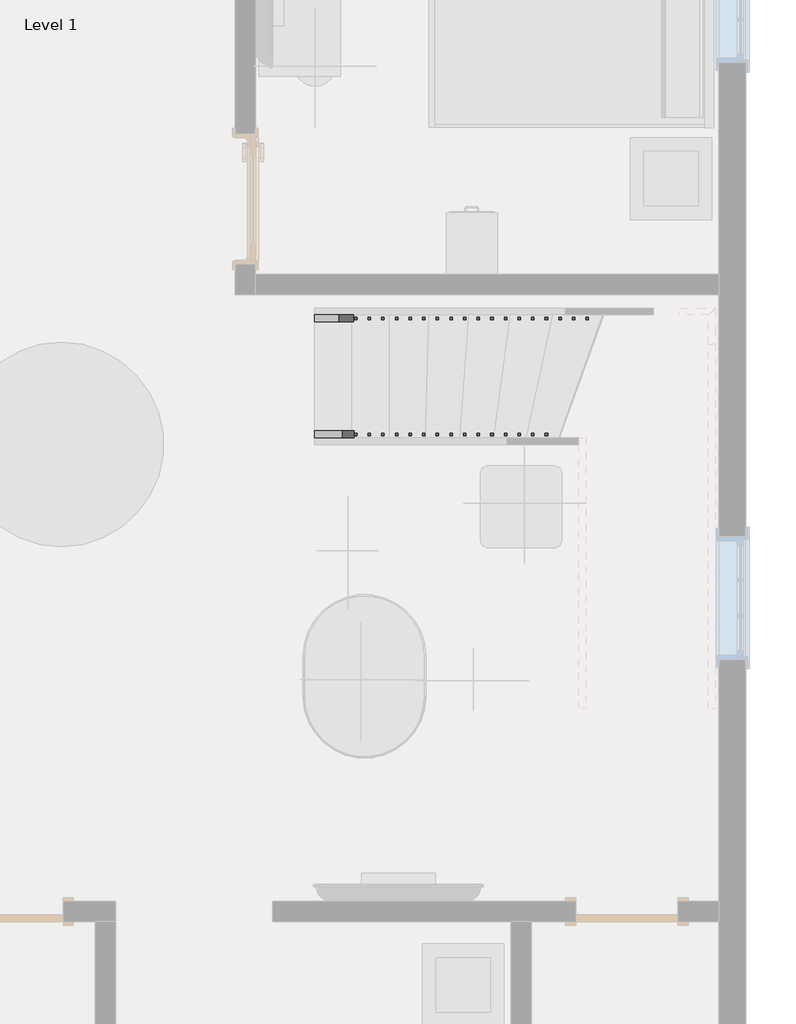
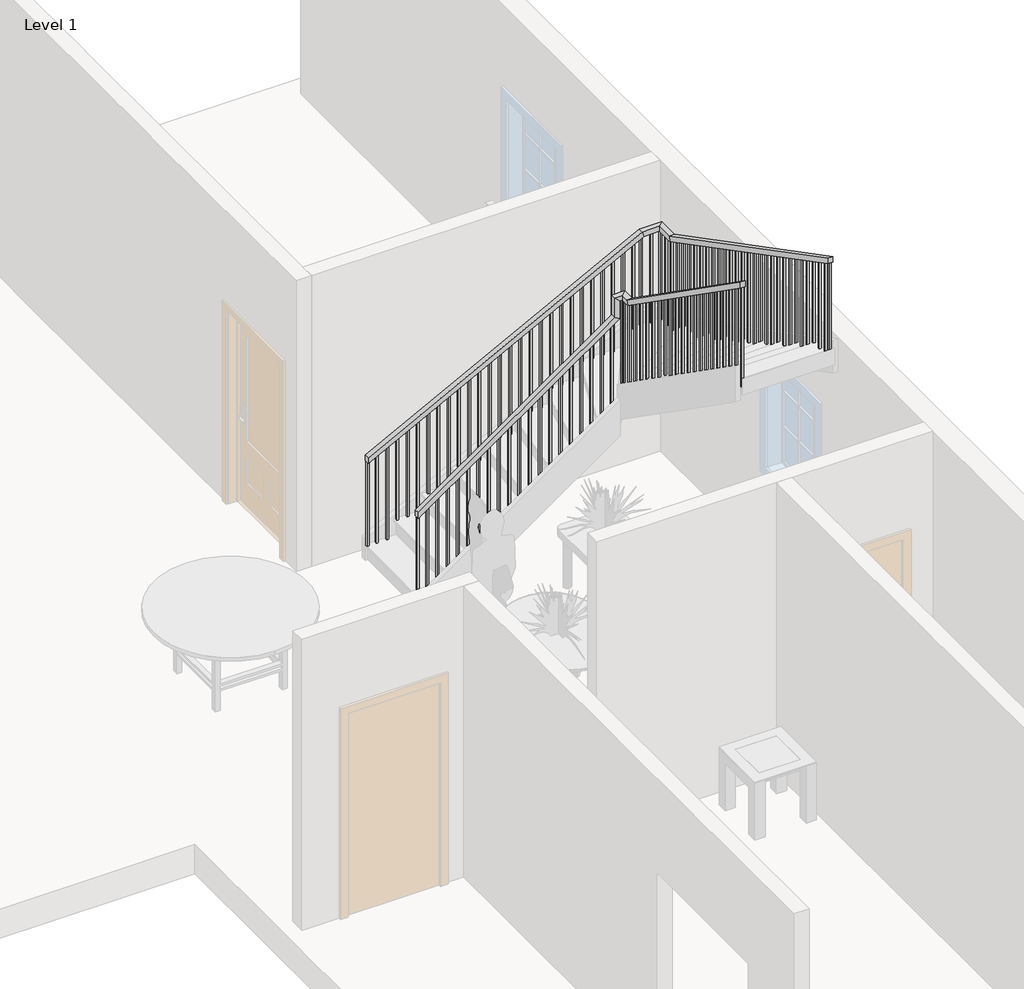
# One storey, part 3 of 4: 2 railings.
"""IFC4 building model written with IfcOpenShell, lengths in millimetres."""

from ifc_helpers import new_model, si_unit, frame, origin, place, context, project, spatial, polyline, outline, extrude, faceted_brep, element, save

model = new_model("IFC4")

# Units and contexts
model_context = context("Model", 3, world=origin())
ifc_project = project(units=[si_unit("LENGTHUNIT", "METRE", prefix="MILLI")], contexts=[model_context])

# Site, building, storey
site = spatial("IfcSite", under=ifc_project)
building = spatial("IfcBuilding", under=site)
storey = spatial("IfcBuildingStorey", under=building, Name="Level 1", Elevation=0.0)

# Railings
placement = place(None, origin())
element("IfcRailing", 1, ObjectType="Handrail - Rectangular", at=placement, inside=storey, context=model_context, shape_type="SolidModel", body=[
    faceted_brep([(-5670.2346501, 6461.8271763, 1057.2428855), (-5670.2346501, 6461.8271763, 995.2081543), (-5670.2346501, 6411.0271763, 995.2081543), (-5670.2346501, 6411.0271763, 1057.2428855), (-3724.8976606, 6461.8271763, 2420.6761173), (-3674.0976606, 6461.8271763, 2394.2457099), (-3674.0976606, 6411.0271763, 2394.2457099), (-3724.8976606, 6411.0271763, 2420.6761173), (-3724.8976606, 6461.8271763, 2625.457216), (-3674.0976606, 6461.8271763, 2574.657216), (-3674.0976606, 6411.0271763, 2574.657216), (-3724.8976606, 6411.0271763, 2625.457216), (-3597.8976606, 6461.8271763, 2625.457216), (-3597.8976606, 6461.8271763, 2574.657216), (-3648.6976606, 6411.0271763, 2574.657216), (-3648.6976606, 6411.0271763, 2625.457216), (-3597.8976606, 6334.8271763, 2625.457216), (-3597.8976606, 6318.7975404, 2574.657216), (-3648.6976606, 6318.7975404, 2574.657216), (-3648.6976606, 6334.8271763, 2625.457216), (-3597.8976606, 4389.4901868, 3988.8904479), (-3648.6976606, 4389.4901868, 3988.8904479), (-3648.6976606, 4389.4901868, 3926.8557166), (-3597.8976606, 4389.4901868, 3926.8557166)], [[[0, 1, 2, 3]], [[1, 0, 4, 5]], [[2, 1, 5, 6]], [[3, 2, 6, 7]], [[0, 3, 7, 4]], [[5, 4, 8, 9]], [[6, 5, 9, 10]], [[7, 6, 10, 11]], [[4, 7, 11, 8]], [[9, 8, 12, 13]], [[10, 9, 13, 14]], [[11, 10, 14, 15]], [[8, 11, 15, 12]], [[13, 12, 16, 17]], [[14, 13, 17, 18]], [[15, 14, 18, 19]], [[12, 15, 19, 16]], [[20, 21, 22, 23]], [[17, 16, 20, 23]], [[18, 17, 23, 22]], [[19, 18, 22, 21]], [[16, 19, 21, 20]]]),
    extrude(outline(polyline([(4394.9021763, 3923.0626019), (4413.9521763, 3909.7109805), (4413.9521763, 2878.6666667), (4394.9021763, 2878.6666667), (4394.9021763, 3923.0626019)])), frame((-3632.8226606, 0.0, 0.0), z_axis=(1.0, 0.0, 0.0), x_axis=(0.0, 1.0, 0.0)), (0.0, 0.0, 1.0), 19.05),
    extrude(outline(polyline([(4496.5021763, 3851.8539542), (4515.5521763, 3838.5023328), (4515.5521763, 2878.6666667), (4496.5021763, 2878.6666667), (4496.5021763, 3851.8539542)])), frame((-3632.8226606, 0.0, 0.0), z_axis=(1.0, 0.0, 0.0), x_axis=(0.0, 1.0, 0.0)), (0.0, 0.0, 1.0), 19.05),
    extrude(outline(polyline([(4598.1021763, 3780.7235858), (4617.1521763, 3767.3719643), (4617.1521763, 2878.6666667), (4598.1021763, 2878.6666667), (4598.1021763, 3780.7235858)])), frame((-3632.8226606, 0.0, 0.0), z_axis=(1.0, 0.0, 0.0), x_axis=(0.0, 1.0, 0.0)), (0.0, 0.0, 1.0), 19.05),
    extrude(outline(polyline([(4699.7021763, 3709.514938), (4718.7521763, 3696.1633166), (4718.7521763, 2709.3333333), (4699.7021763, 2709.3333333), (4699.7021763, 3709.514938)])), frame((-3632.8226606, 0.0, 0.0), z_axis=(1.0, 0.0, 0.0), x_axis=(0.0, 1.0, 0.0)), (0.0, 0.0, 1.0), 19.05),
    extrude(outline(polyline([(4801.3021763, 3638.3062903), (4820.3521763, 3624.9546689), (4820.3521763, 2709.3333333), (4801.3021763, 2709.3333333), (4801.3021763, 3638.3062903)])), frame((-3632.8226606, 0.0, 0.0), z_axis=(1.0, 0.0, 0.0), x_axis=(0.0, 1.0, 0.0)), (0.0, 0.0, 1.0), 19.05),
    extrude(outline(polyline([(4902.9021763, 3567.0193634), (4921.9521763, 3553.667742), (4921.9521763, 2709.3333333), (4902.9021763, 2709.3333333), (4902.9021763, 3567.0193634)])), frame((-3632.8226606, 0.0, 0.0), z_axis=(1.0, 0.0, 0.0), x_axis=(0.0, 1.0, 0.0)), (0.0, 0.0, 1.0), 19.05),
    extrude(outline(polyline([(5004.5021763, 3495.8889949), (5023.5521763, 3482.5373735), (5023.5521763, 2540.0), (5004.5021763, 2540.0), (5004.5021763, 3495.8889949)])), frame((-3632.8226606, 0.0, 0.0), z_axis=(1.0, 0.0, 0.0), x_axis=(0.0, 1.0, 0.0)), (0.0, 0.0, 1.0), 19.05),
    extrude(outline(polyline([(5106.1021763, 3424.602068), (5125.1521763, 3411.2504466), (5125.1521763, 2540.0), (5106.1021763, 2540.0), (5106.1021763, 3424.602068)])), frame((-3632.8226606, 0.0, 0.0), z_axis=(1.0, 0.0, 0.0), x_axis=(0.0, 1.0, 0.0)), (0.0, 0.0, 1.0), 19.05),
    extrude(outline(polyline([(5207.7021763, 3353.4716995), (5226.7521763, 3340.1200781), (5226.7521763, 2370.6666667), (5207.7021763, 2370.6666667), (5207.7021763, 3353.4716995)])), frame((-3632.8226606, 0.0, 0.0), z_axis=(1.0, 0.0, 0.0), x_axis=(0.0, 1.0, 0.0)), (0.0, 0.0, 1.0), 19.05),
    extrude(outline(polyline([(5309.3021763, 3282.1847726), (5328.3521763, 3268.8331511), (5328.3521763, 2370.6666667), (5309.3021763, 2370.6666667), (5309.3021763, 3282.1847726)])), frame((-3632.8226606, 0.0, 0.0), z_axis=(1.0, 0.0, 0.0), x_axis=(0.0, 1.0, 0.0)), (0.0, 0.0, 1.0), 19.05),
    extrude(outline(polyline([(5410.9021763, 3210.9761249), (5429.9521763, 3197.6245034), (5429.9521763, 2370.6666667), (5410.9021763, 2370.6666667), (5410.9021763, 3210.9761249)])), frame((-3632.8226606, 0.0, 0.0), z_axis=(1.0, 0.0, 0.0), x_axis=(0.0, 1.0, 0.0)), (0.0, 0.0, 1.0), 19.05),
    extrude(outline(polyline([(5512.5021763, 3139.8457564), (5531.5521763, 3126.494135), (5531.5521763, 2201.3333333), (5512.5021763, 2201.3333333), (5512.5021763, 3139.8457564)])), frame((-3632.8226606, 0.0, 0.0), z_axis=(1.0, 0.0, 0.0), x_axis=(0.0, 1.0, 0.0)), (0.0, 0.0, 1.0), 19.05),
    extrude(outline(polyline([(5614.1021763, 3068.5588295), (5633.1521763, 3055.207208), (5633.1521763, 2201.3333333), (5614.1021763, 2201.3333333), (5614.1021763, 3068.5588295)])), frame((-3632.8226606, 0.0, 0.0), z_axis=(1.0, 0.0, 0.0), x_axis=(0.0, 1.0, 0.0)), (0.0, 0.0, 1.0), 19.05),
    extrude(outline(polyline([(5715.7021763, 2997.3501818), (5734.7521763, 2983.9985603), (5734.7521763, 2201.3333333), (5715.7021763, 2201.3333333), (5715.7021763, 2997.3501818)])), frame((-3632.8226606, 0.0, 0.0), z_axis=(1.0, 0.0, 0.0), x_axis=(0.0, 1.0, 0.0)), (0.0, 0.0, 1.0), 19.05),
    extrude(outline(polyline([(5817.3021763, 2926.1415341), (5836.3521763, 2912.7899126), (5836.3521763, 2032.0), (5817.3021763, 2032.0), (5817.3021763, 2926.1415341)])), frame((-3632.8226606, 0.0, 0.0), z_axis=(1.0, 0.0, 0.0), x_axis=(0.0, 1.0, 0.0)), (0.0, 0.0, 1.0), 19.05),
    extrude(outline(polyline([(5918.9021763, 2854.9328864), (5937.9521763, 2841.5812649), (5937.9521763, 2032.0), (5918.9021763, 2032.0), (5918.9021763, 2854.9328864)])), frame((-3632.8226606, 0.0, 0.0), z_axis=(1.0, 0.0, 0.0), x_axis=(0.0, 1.0, 0.0)), (0.0, 0.0, 1.0), 19.05),
    extrude(outline(polyline([(6020.5021763, 2783.8025179), (6039.5521763, 2770.4508964), (6039.5521763, 1862.6666667), (6020.5021763, 1862.6666667), (6020.5021763, 2783.8025179)])), frame((-3632.8226606, 0.0, 0.0), z_axis=(1.0, 0.0, 0.0), x_axis=(0.0, 1.0, 0.0)), (0.0, 0.0, 1.0), 19.05),
    extrude(outline(polyline([(6122.1021763, 2712.515591), (6141.1521763, 2699.1639695), (6141.1521763, 1862.6666667), (6122.1021763, 1862.6666667), (6122.1021763, 2712.515591)])), frame((-3632.8226606, 0.0, 0.0), z_axis=(1.0, 0.0, 0.0), x_axis=(0.0, 1.0, 0.0)), (0.0, 0.0, 1.0), 19.05),
    extrude(outline(polyline([(6223.7021763, 2641.3852225), (6242.7521763, 2628.033601), (6242.7521763, 1693.3333333), (6223.7021763, 1693.3333333), (6223.7021763, 2641.3852225)])), frame((-3632.8226606, 0.0, 0.0), z_axis=(1.0, 0.0, 0.0), x_axis=(0.0, 1.0, 0.0)), (0.0, 0.0, 1.0), 19.05),
    extrude(outline(polyline([(-3632.8226606, 6344.3521763), (-3613.7726606, 6344.3521763), (-3613.7726606, 6325.3021763), (-3632.8226606, 6325.3021763), (-3632.8226606, 6344.3521763)])), frame((0.0, 0.0, 1693.3333333), z_axis=(0.0, 0.0, 1.0), x_axis=(1.0, 0.0, 0.0)), (0.0, 0.0, 1.0), 881.3238827),
    extrude(outline(polyline([(-3647.7596501, 6426.9021763), (-3647.7596501, 6445.9521763), (-3628.7096501, 6445.9521763), (-3628.7096501, 6426.9021763), (-3647.7596501, 6426.9021763)])), frame((0.0, 0.0, 1524.0), z_axis=(0.0, 0.0, 1.0), x_axis=(1.0, 0.0, 0.0)), (0.0, 0.0, 1.0), 1050.657216),
    extrude(outline(polyline([(2354.8482714, -3730.3096501), (2341.4966499, -3749.3596501), (1354.6666667, -3749.3596501), (1354.6666667, -3730.3096501), (2354.8482714, -3730.3096501)])), frame((0.0, 6426.9021763, 0.0), z_axis=(0.0, 1.0, 0.0), x_axis=(0.0, 0.0, 1.0)), (0.0, 0.0, 1.0), 19.05),
    extrude(outline(polyline([(2283.6396237, -3831.9096501), (2270.2880022, -3850.9596501), (1354.6666667, -3850.9596501), (1354.6666667, -3831.9096501), (2283.6396237, -3831.9096501)])), frame((0.0, 6426.9021763, 0.0), z_axis=(0.0, 1.0, 0.0), x_axis=(0.0, 0.0, 1.0)), (0.0, 0.0, 1.0), 19.05),
    extrude(outline(polyline([(2212.430976, -3933.5096501), (2199.0793545, -3952.5596501), (1185.3333333, -3952.5596501), (1185.3333333, -3933.5096501), (2212.430976, -3933.5096501)])), frame((0.0, 6426.9021763, 0.0), z_axis=(0.0, 1.0, 0.0), x_axis=(0.0, 0.0, 1.0)), (0.0, 0.0, 1.0), 19.05),
    extrude(outline(polyline([(2141.2223283, -4035.1096501), (2127.8707068, -4054.1596501), (1185.3333333, -4054.1596501), (1185.3333333, -4035.1096501), (2141.2223283, -4035.1096501)])), frame((0.0, 6426.9021763, 0.0), z_axis=(0.0, 1.0, 0.0), x_axis=(0.0, 0.0, 1.0)), (0.0, 0.0, 1.0), 19.05),
    extrude(outline(polyline([(2070.0136806, -4136.7096501), (2056.6620591, -4155.7596501), (1016.0, -4155.7596501), (1016.0, -4136.7096501), (2070.0136806, -4136.7096501)])), frame((0.0, 6426.9021763, 0.0), z_axis=(0.0, 1.0, 0.0), x_axis=(0.0, 0.0, 1.0)), (0.0, 0.0, 1.0), 19.05),
    extrude(outline(polyline([(1998.8050329, -4238.3096501), (1985.4534114, -4257.3596501), (1016.0, -4257.3596501), (1016.0, -4238.3096501), (1998.8050329, -4238.3096501)])), frame((0.0, 6426.9021763, 0.0), z_axis=(0.0, 1.0, 0.0), x_axis=(0.0, 0.0, 1.0)), (0.0, 0.0, 1.0), 19.05),
    extrude(outline(polyline([(1927.5963851, -4339.9096501), (1914.2447637, -4358.9596501), (846.6666667, -4358.9596501), (846.6666667, -4339.9096501), (1927.5963851, -4339.9096501)])), frame((0.0, 6426.9021763, 0.0), z_axis=(0.0, 1.0, 0.0), x_axis=(0.0, 0.0, 1.0)), (0.0, 0.0, 1.0), 19.05),
    extrude(outline(polyline([(1856.3877374, -4441.5096501), (1843.036116, -4460.5596501), (846.6666667, -4460.5596501), (846.6666667, -4441.5096501), (1856.3877374, -4441.5096501)])), frame((0.0, 6426.9021763, 0.0), z_axis=(0.0, 1.0, 0.0), x_axis=(0.0, 0.0, 1.0)), (0.0, 0.0, 1.0), 19.05),
    extrude(outline(polyline([(1785.1790897, -4543.1096501), (1771.8274683, -4562.1596501), (846.6666667, -4562.1596501), (846.6666667, -4543.1096501), (1785.1790897, -4543.1096501)])), frame((0.0, 6426.9021763, 0.0), z_axis=(0.0, 1.0, 0.0), x_axis=(0.0, 0.0, 1.0)), (0.0, 0.0, 1.0), 19.05),
    extrude(outline(polyline([(1713.970442, -4644.7096501), (1700.6188206, -4663.7596501), (677.3333333, -4663.7596501), (677.3333333, -4644.7096501), (1713.970442, -4644.7096501)])), frame((0.0, 6426.9021763, 0.0), z_axis=(0.0, 1.0, 0.0), x_axis=(0.0, 0.0, 1.0)), (0.0, 0.0, 1.0), 19.05),
    extrude(outline(polyline([(1642.7617943, -4746.3096501), (1629.4101729, -4765.3596501), (677.3333333, -4765.3596501), (677.3333333, -4746.3096501), (1642.7617943, -4746.3096501)])), frame((0.0, 6426.9021763, 0.0), z_axis=(0.0, 1.0, 0.0), x_axis=(0.0, 0.0, 1.0)), (0.0, 0.0, 1.0), 19.05),
    extrude(outline(polyline([(1571.5531466, -4847.9096501), (1558.2015252, -4866.9596501), (508.0, -4866.9596501), (508.0, -4847.9096501), (1571.5531466, -4847.9096501)])), frame((0.0, 6426.9021763, 0.0), z_axis=(0.0, 1.0, 0.0), x_axis=(0.0, 0.0, 1.0)), (0.0, 0.0, 1.0), 19.05),
    extrude(outline(polyline([(1500.3444989, -4949.5096501), (1486.9928775, -4968.5596501), (508.0, -4968.5596501), (508.0, -4949.5096501), (1500.3444989, -4949.5096501)])), frame((0.0, 6426.9021763, 0.0), z_axis=(0.0, 1.0, 0.0), x_axis=(0.0, 0.0, 1.0)), (0.0, 0.0, 1.0), 19.05),
    extrude(outline(polyline([(1429.1358512, -5051.1096501), (1415.7842298, -5070.1596501), (508.0, -5070.1596501), (508.0, -5051.1096501), (1429.1358512, -5051.1096501)])), frame((0.0, 6426.9021763, 0.0), z_axis=(0.0, 1.0, 0.0), x_axis=(0.0, 0.0, 1.0)), (0.0, 0.0, 1.0), 19.05),
    extrude(outline(polyline([(1357.9272035, -5152.7096501), (1344.5755821, -5171.7596501), (338.6666667, -5171.7596501), (338.6666667, -5152.7096501), (1357.9272035, -5152.7096501)])), frame((0.0, 6426.9021763, 0.0), z_axis=(0.0, 1.0, 0.0), x_axis=(0.0, 0.0, 1.0)), (0.0, 0.0, 1.0), 19.05),
    extrude(outline(polyline([(1286.7185558, -5254.3096501), (1273.3669344, -5273.3596501), (338.6666667, -5273.3596501), (338.6666667, -5254.3096501), (1286.7185558, -5254.3096501)])), frame((0.0, 6426.9021763, 0.0), z_axis=(0.0, 1.0, 0.0), x_axis=(0.0, 0.0, 1.0)), (0.0, 0.0, 1.0), 19.05),
    extrude(outline(polyline([(1215.5099081, -5355.9096501), (1202.1582867, -5374.9596501), (338.6666667, -5374.9596501), (338.6666667, -5355.9096501), (1215.5099081, -5355.9096501)])), frame((0.0, 6426.9021763, 0.0), z_axis=(0.0, 1.0, 0.0), x_axis=(0.0, 0.0, 1.0)), (0.0, 0.0, 1.0), 19.05),
    extrude(outline(polyline([(1144.2229812, -5457.5096501), (1130.8713597, -5476.5596501), (169.3333333, -5476.5596501), (169.3333333, -5457.5096501), (1144.2229812, -5457.5096501)])), frame((0.0, 6426.9021763, 0.0), z_axis=(0.0, 1.0, 0.0), x_axis=(0.0, 0.0, 1.0)), (0.0, 0.0, 1.0), 19.05),
    extrude(outline(polyline([(1073.0926127, -5559.1096501), (1059.7409912, -5578.1596501), (169.3333333, -5578.1596501), (169.3333333, -5559.1096501), (1073.0926127, -5559.1096501)])), frame((0.0, 6426.9021763, 0.0), z_axis=(0.0, 1.0, 0.0), x_axis=(0.0, 0.0, 1.0)), (0.0, 0.0, 1.0), 19.05),
    extrude(outline(polyline([(-3632.8226606, 6445.9521763), (-3613.7726606, 6445.9521763), (-3613.7726606, 6426.9021763), (-3632.8226606, 6426.9021763), (-3632.8226606, 6445.9521763)])), frame((0.0, 0.0, 1524.0), z_axis=(0.0, 0.0, 1.0), x_axis=(1.0, 0.0, 0.0)), (0.0, 0.0, 1.0), 1050.657216),
    extrude(outline(polyline([(4389.4901868, 3926.8557166), (4408.5401868, 3913.5040952), (4408.5401868, 2878.6666667), (4389.4901868, 2878.6666667), (4389.4901868, 3926.8557166)])), frame((-3632.8226606, 0.0, 0.0), z_axis=(1.0, 0.0, 0.0), x_axis=(0.0, 1.0, 0.0)), (0.0, 0.0, 1.0), 19.05),
    extrude(outline(polyline([(1008.5597757, -5651.1846501), (995.2081543, -5670.2346501), (169.3333333, -5670.2346501), (169.3333333, -5651.1846501), (1008.5597757, -5651.1846501)])), frame((0.0, 6426.9021763, 0.0), z_axis=(0.0, 1.0, 0.0), x_axis=(0.0, 0.0, 1.0)), (0.0, 0.0, 1.0), 19.05),
])
element("IfcRailing", 2, ObjectType="Handrail - Rectangular", at=placement, inside=storey, context=model_context, shape_type="SolidModel", body=[
    faceted_brep([(-5670.2346501, 7325.4271763, 1107.5448574), (-5670.2346501, 7325.4271763, 1050.2675251), (-5670.2346501, 7274.6271763, 1050.2675251), (-5670.2346501, 7274.6271763, 1107.5448574), (-2952.4510037, 7325.4271763, 2523.0666667), (-2940.0146092, 7325.4271763, 2472.2666667), (-2940.0146092, 7274.6271763, 2472.2666667), (-2952.4510037, 7274.6271763, 2523.0666667), (-2734.2976606, 7325.4271763, 2523.0666667), (-2734.2976606, 7325.4271763, 2472.2666667), (-2785.0976606, 7274.6271763, 2472.2666667), (-2785.0976606, 7274.6271763, 2523.0666667), (-2734.2976606, 7107.2738332, 2523.0666667), (-2734.2976606, 7094.8374386, 2472.2666667), (-2785.0976606, 7094.8374386, 2472.2666667), (-2785.0976606, 7107.2738332, 2523.0666667), (-2734.2976606, 4389.4901868, 3938.588476), (-2785.0976606, 4389.4901868, 3938.588476), (-2785.0976606, 4389.4901868, 3881.3111437), (-2734.2976606, 4389.4901868, 3881.3111437)], [[[0, 1, 2, 3]], [[1, 0, 4, 5]], [[2, 1, 5, 6]], [[3, 2, 6, 7]], [[0, 3, 7, 4]], [[5, 4, 8, 9]], [[6, 5, 9, 10]], [[7, 6, 10, 11]], [[4, 7, 11, 8]], [[9, 8, 12, 13]], [[10, 9, 13, 14]], [[11, 10, 14, 15]], [[8, 11, 15, 12]], [[16, 17, 18, 19]], [[13, 12, 16, 19]], [[14, 13, 19, 18]], [[15, 14, 18, 17]], [[12, 15, 17, 16]]]),
    extrude(outline(polyline([(4475.1988332, 3836.6652459), (4475.1988332, 2878.6666667), (4456.1488332, 2878.6666667), (4456.1488332, 3846.5871875), (4475.1988332, 3836.6652459)])), frame((-2769.2226606, 0.0, 0.0), z_axis=(1.0, 0.0, 0.0), x_axis=(0.0, 1.0, 0.0)), (0.0, 0.0, 1.0), 19.05),
    extrude(outline(polyline([(4576.7988332, 3783.7539027), (4576.7988332, 2878.6666667), (4557.7488332, 2878.6666667), (4557.7488332, 3793.6758443), (4576.7988332, 3783.7539027)])), frame((-2769.2226606, 0.0, 0.0), z_axis=(1.0, 0.0, 0.0), x_axis=(0.0, 1.0, 0.0)), (0.0, 0.0, 1.0), 19.05),
    extrude(outline(polyline([(4678.3988332, 3730.8368812), (4678.3988332, 2878.6751842), (4659.3488332, 2878.6751842), (4659.3488332, 3740.7588227), (4678.3988332, 3730.8368812)])), frame((-2769.2226606, 0.0, 0.0), z_axis=(1.0, 0.0, 0.0), x_axis=(0.0, 1.0, 0.0)), (0.0, 0.0, 1.0), 19.05),
    extrude(outline(polyline([(4779.9988332, 3677.9141812), (4779.9988332, 2709.3333333), (4760.9488332, 2709.3333333), (4760.9488332, 3687.8361228), (4779.9988332, 3677.9141812)])), frame((-2769.2226606, 0.0, 0.0), z_axis=(1.0, 0.0, 0.0), x_axis=(0.0, 1.0, 0.0)), (0.0, 0.0, 1.0), 19.05),
    extrude(outline(polyline([(4881.5988332, 3624.9971597), (4881.5988332, 2709.3333333), (4862.5488332, 2709.3333333), (4862.5488332, 3634.9191012), (4881.5988332, 3624.9971597)])), frame((-2769.2226606, 0.0, 0.0), z_axis=(1.0, 0.0, 0.0), x_axis=(0.0, 1.0, 0.0)), (0.0, 0.0, 1.0), 19.05),
    extrude(outline(polyline([(4983.1988332, 3572.0801381), (4983.1988332, 2540.0), (4964.1488332, 2540.0), (4964.1488332, 3582.0020796), (4983.1988332, 3572.0801381)])), frame((-2769.2226606, 0.0, 0.0), z_axis=(1.0, 0.0, 0.0), x_axis=(0.0, 1.0, 0.0)), (0.0, 0.0, 1.0), 19.05),
    extrude(outline(polyline([(5084.7988332, 3519.1631165), (5084.7988332, 2540.0), (5065.7488332, 2540.0), (5065.7488332, 3529.0850581), (5084.7988332, 3519.1631165)])), frame((-2769.2226606, 0.0, 0.0), z_axis=(1.0, 0.0, 0.0), x_axis=(0.0, 1.0, 0.0)), (0.0, 0.0, 1.0), 19.05),
    extrude(outline(polyline([(5186.3988332, 3466.246095), (5186.3988332, 2540.0), (5167.3488332, 2540.0), (5167.3488332, 3476.1680365), (5186.3988332, 3466.246095)])), frame((-2769.2226606, 0.0, 0.0), z_axis=(1.0, 0.0, 0.0), x_axis=(0.0, 1.0, 0.0)), (0.0, 0.0, 1.0), 19.05),
    extrude(outline(polyline([(5287.9988332, 3413.3347518), (5287.9988332, 2370.6666667), (5268.9488332, 2370.6666667), (5268.9488332, 3423.2566933), (5287.9988332, 3413.3347518)])), frame((-2769.2226606, 0.0, 0.0), z_axis=(1.0, 0.0, 0.0), x_axis=(0.0, 1.0, 0.0)), (0.0, 0.0, 1.0), 19.05),
    extrude(outline(polyline([(5389.5988332, 3360.4120518), (5389.5988332, 2370.6666667), (5370.5488332, 2370.6666667), (5370.5488332, 3370.3339934), (5389.5988332, 3360.4120518)])), frame((-2769.2226606, 0.0, 0.0), z_axis=(1.0, 0.0, 0.0), x_axis=(0.0, 1.0, 0.0)), (0.0, 0.0, 1.0), 19.05),
    extrude(outline(polyline([(5491.1988332, 3307.4950303), (5491.1988332, 2370.6666667), (5472.1488332, 2370.6666667), (5472.1488332, 3317.4169718), (5491.1988332, 3307.4950303)])), frame((-2769.2226606, 0.0, 0.0), z_axis=(1.0, 0.0, 0.0), x_axis=(0.0, 1.0, 0.0)), (0.0, 0.0, 1.0), 19.05),
    extrude(outline(polyline([(5592.7988332, 3254.5836871), (5592.7988332, 2201.3333333), (5573.7488332, 2201.3333333), (5573.7488332, 3264.5056286), (5592.7988332, 3254.5836871)])), frame((-2769.2226606, 0.0, 0.0), z_axis=(1.0, 0.0, 0.0), x_axis=(0.0, 1.0, 0.0)), (0.0, 0.0, 1.0), 19.05),
    extrude(outline(polyline([(5694.3988332, 3201.6666655), (5694.3988332, 2201.3333333), (5675.3488332, 2201.3333333), (5675.3488332, 3211.5886071), (5694.3988332, 3201.6666655)])), frame((-2769.2226606, 0.0, 0.0), z_axis=(1.0, 0.0, 0.0), x_axis=(0.0, 1.0, 0.0)), (0.0, 0.0, 1.0), 19.05),
    extrude(outline(polyline([(5795.9988332, 3148.749644), (5795.9988332, 2201.3333333), (5776.9488332, 2201.3333333), (5776.9488332, 3158.6715855), (5795.9988332, 3148.749644)])), frame((-2769.2226606, 0.0, 0.0), z_axis=(1.0, 0.0, 0.0), x_axis=(0.0, 1.0, 0.0)), (0.0, 0.0, 1.0), 19.05),
    extrude(outline(polyline([(5897.5988332, 3095.8326224), (5897.5988332, 2032.0), (5878.5488332, 2032.0), (5878.5488332, 3105.7545639), (5897.5988332, 3095.8326224)])), frame((-2769.2226606, 0.0, 0.0), z_axis=(1.0, 0.0, 0.0), x_axis=(0.0, 1.0, 0.0)), (0.0, 0.0, 1.0), 19.05),
    extrude(outline(polyline([(5999.1988332, 3042.9156008), (5999.1988332, 2032.0), (5980.1488332, 2032.0), (5980.1488332, 3052.8375424), (5999.1988332, 3042.9156008)])), frame((-2769.2226606, 0.0, 0.0), z_axis=(1.0, 0.0, 0.0), x_axis=(0.0, 1.0, 0.0)), (0.0, 0.0, 1.0), 19.05),
    extrude(outline(polyline([(6100.7988332, 2989.9985793), (6100.7988332, 2032.0), (6081.7488332, 2032.0), (6081.7488332, 2999.9205208), (6100.7988332, 2989.9985793)])), frame((-2769.2226606, 0.0, 0.0), z_axis=(1.0, 0.0, 0.0), x_axis=(0.0, 1.0, 0.0)), (0.0, 0.0, 1.0), 19.05),
    extrude(outline(polyline([(6202.3988332, 2937.0815577), (6202.3988332, 1862.6666667), (6183.3488332, 1862.6666667), (6183.3488332, 2947.0034992), (6202.3988332, 2937.0815577)])), frame((-2769.2226606, 0.0, 0.0), z_axis=(1.0, 0.0, 0.0), x_axis=(0.0, 1.0, 0.0)), (0.0, 0.0, 1.0), 19.05),
    extrude(outline(polyline([(6303.9988332, 2884.1645361), (6303.9988332, 1862.6666667), (6284.9488332, 1862.6666667), (6284.9488332, 2894.0864777), (6303.9988332, 2884.1645361)])), frame((-2769.2226606, 0.0, 0.0), z_axis=(1.0, 0.0, 0.0), x_axis=(0.0, 1.0, 0.0)), (0.0, 0.0, 1.0), 19.05),
    extrude(outline(polyline([(6405.5988332, 2831.2475146), (6405.5988332, 1862.6666667), (6386.5488332, 1862.6666667), (6386.5488332, 2841.1694561), (6405.5988332, 2831.2475146)])), frame((-2769.2226606, 0.0, 0.0), z_axis=(1.0, 0.0, 0.0), x_axis=(0.0, 1.0, 0.0)), (0.0, 0.0, 1.0), 19.05),
    extrude(outline(polyline([(6507.1988332, 2778.330493), (6507.1988332, 1862.6666667), (6488.1488332, 1862.6666667), (6488.1488332, 2788.2524345), (6507.1988332, 2778.330493)])), frame((-2769.2226606, 0.0, 0.0), z_axis=(1.0, 0.0, 0.0), x_axis=(0.0, 1.0, 0.0)), (0.0, 0.0, 1.0), 19.05),
    extrude(outline(polyline([(6608.7988332, 2725.4134714), (6608.7988332, 1693.3333333), (6589.7488332, 1693.3333333), (6589.7488332, 2735.335413), (6608.7988332, 2725.4134714)])), frame((-2769.2226606, 0.0, 0.0), z_axis=(1.0, 0.0, 0.0), x_axis=(0.0, 1.0, 0.0)), (0.0, 0.0, 1.0), 19.05),
    extrude(outline(polyline([(6710.3988332, 2672.4964499), (6710.3988332, 1693.3333333), (6691.3488332, 1693.3333333), (6691.3488332, 2682.4183914), (6710.3988332, 2672.4964499)])), frame((-2769.2226606, 0.0, 0.0), z_axis=(1.0, 0.0, 0.0), x_axis=(0.0, 1.0, 0.0)), (0.0, 0.0, 1.0), 19.05),
    extrude(outline(polyline([(6811.9988332, 2619.5794283), (6811.9988332, 1693.3333333), (6792.9488332, 1693.3333333), (6792.9488332, 2629.5013699), (6811.9988332, 2619.5794283)])), frame((-2769.2226606, 0.0, 0.0), z_axis=(1.0, 0.0, 0.0), x_axis=(0.0, 1.0, 0.0)), (0.0, 0.0, 1.0), 19.05),
    extrude(outline(polyline([(6913.5988332, 2566.6624067), (6913.5988332, 1693.3333333), (6894.5488332, 1693.3333333), (6894.5488332, 2576.5843483), (6913.5988332, 2566.6624067)])), frame((-2769.2226606, 0.0, 0.0), z_axis=(1.0, 0.0, 0.0), x_axis=(0.0, 1.0, 0.0)), (0.0, 0.0, 1.0), 19.05),
    extrude(outline(polyline([(7015.1988332, 2513.7453852), (7015.1988332, 1524.0), (6996.1488332, 1524.0), (6996.1488332, 2523.6673267), (7015.1988332, 2513.7453852)])), frame((-2769.2226606, 0.0, 0.0), z_axis=(1.0, 0.0, 0.0), x_axis=(0.0, 1.0, 0.0)), (0.0, 0.0, 1.0), 19.05),
    extrude(outline(polyline([(-2750.1726606, 7207.9521763), (-2750.1726606, 7188.9021763), (-2769.2226606, 7188.9021763), (-2769.2226606, 7207.9521763), (-2750.1726606, 7207.9521763)])), frame((0.0, 0.0, 1524.0), z_axis=(0.0, 0.0, 1.0), x_axis=(1.0, 0.0, 0.0)), (0.0, 0.0, 1.0), 948.2666667),
    extrude(outline(polyline([(-2860.3760037, 7309.5521763), (-2841.3260037, 7309.5521763), (-2841.3260037, 7290.5021763), (-2860.3760037, 7290.5021763), (-2860.3760037, 7309.5521763)])), frame((0.0, 0.0, 1524.0), z_axis=(0.0, 0.0, 1.0), x_axis=(1.0, 0.0, 0.0)), (0.0, 0.0, 1.0), 948.2666667),
    extrude(outline(polyline([(2421.1434366, -3038.1596501), (1524.0, -3038.1596501), (1524.0, -3019.1096501), (2431.0653782, -3019.1096501), (2421.1434366, -3038.1596501)])), frame((0.0, 7290.5021763, 0.0), z_axis=(0.0, 1.0, 0.0), x_axis=(0.0, 0.0, 1.0)), (0.0, 0.0, 1.0), 19.05),
    extrude(outline(polyline([(2368.2264151, -3139.7596501), (1524.0, -3139.7596501), (1524.0, -3120.7096501), (2378.1483566, -3120.7096501), (2368.2264151, -3139.7596501)])), frame((0.0, 7290.5021763, 0.0), z_axis=(0.0, 1.0, 0.0), x_axis=(0.0, 0.0, 1.0)), (0.0, 0.0, 1.0), 19.05),
    extrude(outline(polyline([(2315.3093935, -3241.3596501), (1354.6666667, -3241.3596501), (1354.6666667, -3222.3096501), (2325.231335, -3222.3096501), (2315.3093935, -3241.3596501)])), frame((0.0, 7290.5021763, 0.0), z_axis=(0.0, 1.0, 0.0), x_axis=(0.0, 0.0, 1.0)), (0.0, 0.0, 1.0), 19.05),
    extrude(outline(polyline([(2262.3923719, -3342.9596501), (1354.6666667, -3342.9596501), (1354.6666667, -3323.9096501), (2272.3143135, -3323.9096501), (2262.3923719, -3342.9596501)])), frame((0.0, 7290.5021763, 0.0), z_axis=(0.0, 1.0, 0.0), x_axis=(0.0, 0.0, 1.0)), (0.0, 0.0, 1.0), 19.05),
    extrude(outline(polyline([(2209.4753504, -3444.5596501), (1354.6666667, -3444.5596501), (1354.6666667, -3425.5096501), (2219.3972919, -3425.5096501), (2209.4753504, -3444.5596501)])), frame((0.0, 7290.5021763, 0.0), z_axis=(0.0, 1.0, 0.0), x_axis=(0.0, 0.0, 1.0)), (0.0, 0.0, 1.0), 19.05),
    extrude(outline(polyline([(2156.5640072, -3546.1596501), (1354.6666667, -3546.1596501), (1354.6666667, -3527.1096501), (2166.4859487, -3527.1096501), (2156.5640072, -3546.1596501)])), frame((0.0, 7290.5021763, 0.0), z_axis=(0.0, 1.0, 0.0), x_axis=(0.0, 0.0, 1.0)), (0.0, 0.0, 1.0), 19.05),
    extrude(outline(polyline([(2103.6413072, -3647.7596501), (1185.3333333, -3647.7596501), (1185.3333333, -3628.7096501), (2113.5632488, -3628.7096501), (2103.6413072, -3647.7596501)])), frame((0.0, 7290.5021763, 0.0), z_axis=(0.0, 1.0, 0.0), x_axis=(0.0, 0.0, 1.0)), (0.0, 0.0, 1.0), 19.05),
    extrude(outline(polyline([(2050.7242857, -3749.3596501), (1185.3333333, -3749.3596501), (1185.3333333, -3730.3096501), (2060.6462272, -3730.3096501), (2050.7242857, -3749.3596501)])), frame((0.0, 7290.5021763, 0.0), z_axis=(0.0, 1.0, 0.0), x_axis=(0.0, 0.0, 1.0)), (0.0, 0.0, 1.0), 19.05),
    extrude(outline(polyline([(1997.8129425, -3850.9596501), (1185.3333333, -3850.9596501), (1185.3333333, -3831.9096501), (2007.734884, -3831.9096501), (1997.8129425, -3850.9596501)])), frame((0.0, 7290.5021763, 0.0), z_axis=(0.0, 1.0, 0.0), x_axis=(0.0, 0.0, 1.0)), (0.0, 0.0, 1.0), 19.05),
    extrude(outline(polyline([(1944.8902425, -3952.5596501), (1016.0, -3952.5596501), (1016.0, -3933.5096501), (1954.8121841, -3933.5096501), (1944.8902425, -3952.5596501)])), frame((0.0, 7290.5021763, 0.0), z_axis=(0.0, 1.0, 0.0), x_axis=(0.0, 0.0, 1.0)), (0.0, 0.0, 1.0), 19.05),
    extrude(outline(polyline([(1891.9788993, -4054.1596501), (1016.0, -4054.1596501), (1016.0, -4035.1096501), (1901.9008409, -4035.1096501), (1891.9788993, -4054.1596501)])), frame((0.0, 7290.5021763, 0.0), z_axis=(0.0, 1.0, 0.0), x_axis=(0.0, 0.0, 1.0)), (0.0, 0.0, 1.0), 19.05),
    extrude(outline(polyline([(1839.0618778, -4155.7596501), (1016.0, -4155.7596501), (1016.0, -4136.7096501), (1848.9838193, -4136.7096501), (1839.0618778, -4155.7596501)])), frame((0.0, 7290.5021763, 0.0), z_axis=(0.0, 1.0, 0.0), x_axis=(0.0, 0.0, 1.0)), (0.0, 0.0, 1.0), 19.05),
    extrude(outline(polyline([(1786.1448562, -4257.3596501), (846.6666667, -4257.3596501), (846.6666667, -4238.3096501), (1796.0667978, -4238.3096501), (1786.1448562, -4257.3596501)])), frame((0.0, 7290.5021763, 0.0), z_axis=(0.0, 1.0, 0.0), x_axis=(0.0, 0.0, 1.0)), (0.0, 0.0, 1.0), 19.05),
    extrude(outline(polyline([(1733.2278347, -4358.9596501), (846.6666667, -4358.9596501), (846.6666667, -4339.9096501), (1743.1497762, -4339.9096501), (1733.2278347, -4358.9596501)])), frame((0.0, 7290.5021763, 0.0), z_axis=(0.0, 1.0, 0.0), x_axis=(0.0, 0.0, 1.0)), (0.0, 0.0, 1.0), 19.05),
    extrude(outline(polyline([(1680.3108131, -4460.5596501), (846.6666667, -4460.5596501), (846.6666667, -4441.5096501), (1690.2327546, -4441.5096501), (1680.3108131, -4460.5596501)])), frame((0.0, 7290.5021763, 0.0), z_axis=(0.0, 1.0, 0.0), x_axis=(0.0, 0.0, 1.0)), (0.0, 0.0, 1.0), 19.05),
    extrude(outline(polyline([(1627.3937915, -4562.1596501), (677.3333333, -4562.1596501), (677.3333333, -4543.1096501), (1637.3157331, -4543.1096501), (1627.3937915, -4562.1596501)])), frame((0.0, 7290.5021763, 0.0), z_axis=(0.0, 1.0, 0.0), x_axis=(0.0, 0.0, 1.0)), (0.0, 0.0, 1.0), 19.05),
    extrude(outline(polyline([(1574.47677, -4663.7596501), (677.3333333, -4663.7596501), (677.3333333, -4644.7096501), (1584.3987115, -4644.7096501), (1574.47677, -4663.7596501)])), frame((0.0, 7290.5021763, 0.0), z_axis=(0.0, 1.0, 0.0), x_axis=(0.0, 0.0, 1.0)), (0.0, 0.0, 1.0), 19.05),
    extrude(outline(polyline([(1521.5597484, -4765.3596501), (677.3333333, -4765.3596501), (677.3333333, -4746.3096501), (1531.4816899, -4746.3096501), (1521.5597484, -4765.3596501)])), frame((0.0, 7290.5021763, 0.0), z_axis=(0.0, 1.0, 0.0), x_axis=(0.0, 0.0, 1.0)), (0.0, 0.0, 1.0), 19.05),
    extrude(outline(polyline([(1468.6427268, -4866.9596501), (508.0, -4866.9596501), (508.0, -4847.9096501), (1478.5646684, -4847.9096501), (1468.6427268, -4866.9596501)])), frame((0.0, 7290.5021763, 0.0), z_axis=(0.0, 1.0, 0.0), x_axis=(0.0, 0.0, 1.0)), (0.0, 0.0, 1.0), 19.05),
    extrude(outline(polyline([(1415.7257053, -4968.5596501), (508.0, -4968.5596501), (508.0, -4949.5096501), (1425.6476468, -4949.5096501), (1415.7257053, -4968.5596501)])), frame((0.0, 7290.5021763, 0.0), z_axis=(0.0, 1.0, 0.0), x_axis=(0.0, 0.0, 1.0)), (0.0, 0.0, 1.0), 19.05),
    extrude(outline(polyline([(1362.8086837, -5070.1596501), (508.0, -5070.1596501), (508.0, -5051.1096501), (1372.7306252, -5051.1096501), (1362.8086837, -5070.1596501)])), frame((0.0, 7290.5021763, 0.0), z_axis=(0.0, 1.0, 0.0), x_axis=(0.0, 0.0, 1.0)), (0.0, 0.0, 1.0), 19.05),
    extrude(outline(polyline([(1309.8916621, -5171.7596501), (338.6666667, -5171.7596501), (338.6666667, -5152.7096501), (1319.8136037, -5152.7096501), (1309.8916621, -5171.7596501)])), frame((0.0, 7290.5021763, 0.0), z_axis=(0.0, 1.0, 0.0), x_axis=(0.0, 0.0, 1.0)), (0.0, 0.0, 1.0), 19.05),
    extrude(outline(polyline([(1256.9746406, -5273.3596501), (338.6666667, -5273.3596501), (338.6666667, -5254.3096501), (1266.8965821, -5254.3096501), (1256.9746406, -5273.3596501)])), frame((0.0, 7290.5021763, 0.0), z_axis=(0.0, 1.0, 0.0), x_axis=(0.0, 0.0, 1.0)), (0.0, 0.0, 1.0), 19.05),
    extrude(outline(polyline([(1204.057619, -5374.9596501), (338.6666667, -5374.9596501), (338.6666667, -5355.9096501), (1213.9795606, -5355.9096501), (1204.057619, -5374.9596501)])), frame((0.0, 7290.5021763, 0.0), z_axis=(0.0, 1.0, 0.0), x_axis=(0.0, 0.0, 1.0)), (0.0, 0.0, 1.0), 19.05),
    extrude(outline(polyline([(1151.1405974, -5476.5596501), (169.3333333, -5476.5596501), (169.3333333, -5457.5096501), (1161.062539, -5457.5096501), (1151.1405974, -5476.5596501)])), frame((0.0, 7290.5021763, 0.0), z_axis=(0.0, 1.0, 0.0), x_axis=(0.0, 0.0, 1.0)), (0.0, 0.0, 1.0), 19.05),
    extrude(outline(polyline([(1098.2235759, -5578.1596501), (169.3333333, -5578.1596501), (169.3333333, -5559.1096501), (1108.1455174, -5559.1096501), (1098.2235759, -5578.1596501)])), frame((0.0, 7290.5021763, 0.0), z_axis=(0.0, 1.0, 0.0), x_axis=(0.0, 0.0, 1.0)), (0.0, 0.0, 1.0), 19.05),
    extrude(outline(polyline([(-2750.1726606, 7116.7988332), (-2750.1726606, 7097.7488332), (-2769.2226606, 7097.7488332), (-2769.2226606, 7116.7988332), (-2750.1726606, 7116.7988332)])), frame((0.0, 0.0, 1524.0), z_axis=(0.0, 0.0, 1.0), x_axis=(1.0, 0.0, 0.0)), (0.0, 0.0, 1.0), 948.2666667),
    extrude(outline(polyline([(-2769.2226606, 7309.5521763), (-2750.1726606, 7309.5521763), (-2750.1726606, 7290.5021763), (-2769.2226606, 7290.5021763), (-2769.2226606, 7309.5521763)])), frame((0.0, 0.0, 1524.0), z_axis=(0.0, 0.0, 1.0), x_axis=(1.0, 0.0, 0.0)), (0.0, 0.0, 1.0), 948.2666667),
    extrude(outline(polyline([(2460.8283636, -2961.9760037), (1524.0, -2961.9760037), (1524.0, -2942.9260037), (2470.7503052, -2942.9260037), (2460.8283636, -2961.9760037)])), frame((0.0, 7290.5021763, 0.0), z_axis=(0.0, 1.0, 0.0), x_axis=(0.0, 0.0, 1.0)), (0.0, 0.0, 1.0), 19.05),
    extrude(outline(polyline([(4408.5401868, 3871.3892021), (4408.5401868, 2878.6666667), (4389.4901868, 2878.6666667), (4389.4901868, 3881.3111437), (4408.5401868, 3871.3892021)])), frame((-2769.2226606, 0.0, 0.0), z_axis=(1.0, 0.0, 0.0), x_axis=(0.0, 1.0, 0.0)), (0.0, 0.0, 1.0), 19.05),
    extrude(outline(polyline([(1050.2675251, -5670.2346501), (169.3333333, -5670.2346501), (169.3333333, -5651.1846501), (1060.1894666, -5651.1846501), (1050.2675251, -5670.2346501)])), frame((0.0, 7290.5021763, 0.0), z_axis=(0.0, 1.0, 0.0), x_axis=(0.0, 0.0, 1.0)), (0.0, 0.0, 1.0), 19.05),
])

save(model, "model.ifc")

# Revit data of these elements
# Type "Handrail - Rectangular"
#   Assembly Code = "C2010400"
#   built-in parameter 1008612 = 0.0416667 (stored number, unit not read)
#   built-in parameter 1008611 = 0.0416667 (stored number, unit not read)
#   built-in parameter 1008609 = 0.333333 (stored number, unit not read)
#   built-in parameter 1008604 = 0.166667 (stored number, unit not read)
#   built-in parameter 1008603 = 0.166667 (stored number, unit not read)
#   Railing Height = 3' - 0"
#   built-in parameter 1008630 = 2
#   built-in parameter 1008610 = 2
#   built-in parameter 1008618 = Baluster - Square : 3/4"
# Elements 1, 2 (IfcRailing, "Handrail - Rectangular")
#   Phase Created = New Construction
